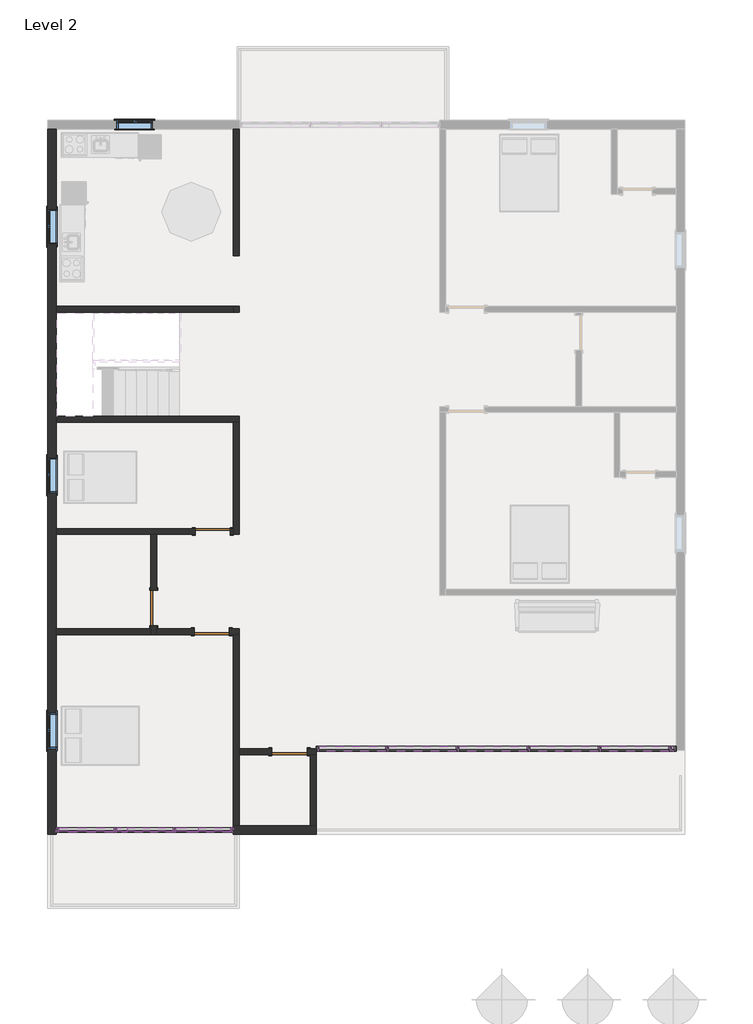
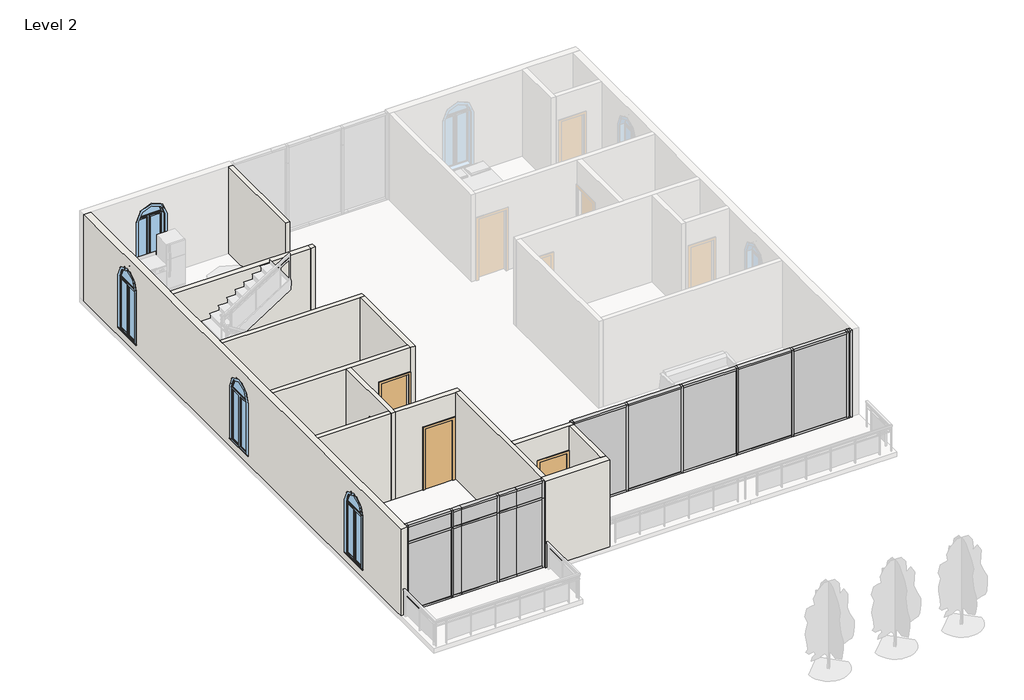
# One storey, part 1 of 3: 42 members, 16 plates, 14 walls, 4 doors, 4 windows.
"""IFC4 building model written with IfcOpenShell, lengths in millimetres."""

from ifc_helpers import new_model, si_unit, frame, origin, place, context, project, spatial, polyline, circle_curve, outline, extrude, faceted_brep, transform, mapped, element, save
from ifc_brep_helpers import plane_surface, revolved_surface, advanced_brep
from components import door_686f89d2, door_16372e1c, member_35f02b64, member_64ee9188, member_6d5c3e5e, member_eaba9652, member_3f395ae9, member_26d67f61, member_f0fea5a5, member_6df10a9f, member_6e77e263, member_ee409385, member_47bfaf8a, member_d2e7e466, member_43f7a5f1, member_c327c56d, member_830eb86c, member_5d67b9fc, member_b5e65c95, member_b3f2e294, member_7db1855a, system_panel_glazed_10fc8cc6, system_panel_glazed_e7b2b8ad, system_panel_glazed_6b5a73aa, system_panel_glazed_adb83807, system_panel_glazed_cd562e5d, system_panel_glazed_a1694ec4, system_panel_glazed_bb2333a0, system_panel_glazed_5dcb8e4e, system_panel_glazed_3760a879, system_panel_glazed_153bb9bb, system_panel_glazed_f2c52b8f, system_panel_glazed_2937bf4c, system_panel_glazed_34036fae, window_e7489165

model = new_model("IFC4")

# Units and contexts
model_context = context("Model", 3, world=origin())
ifc_project = project(units=[si_unit("LENGTHUNIT", "METRE", prefix="MILLI")], contexts=[model_context])

# Site, building, storey
site = spatial("IfcSite", under=ifc_project)
building = spatial("IfcBuilding", under=site)
storey = spatial("IfcBuildingStorey", under=building, Name="Level 2", Elevation=3200.4)

# Doors
placement = place(None, origin())
door_shape = door_686f89d2(model_context)
element("IfcDoor", 1, ObjectType="Single-Flush : 36\" x 84\"", at=placement, inside=storey, context=model_context, shape_type="MappedRepresentation", body=[
    mapped(door_shape, transform((-5050.0707895, -548.4855812, 3200.4), x_axis=(1.0, 0.0, 0.0), y_axis=(0.0, 1.0, 0.0), z_axis=(0.0, 0.0, 1.0))),
])
element("IfcDoor", 2, ObjectType="Single-Flush : 36\" x 84\"", at=placement, inside=storey, context=model_context, shape_type="MappedRepresentation", body=[
    mapped(door_shape, transform((-6548.6707895, 61.1144188, 3200.4), x_axis=(0.0, -1.0, 0.0), y_axis=(1.0, 0.0, 0.0), z_axis=(0.0, 0.0, 1.0))),
])
element("IfcDoor", 3, ObjectType="Single-Flush : 36\" x 84\"", at=placement, inside=storey, context=model_context, shape_type="MappedRepresentation", body=[
    mapped(door_shape, transform((-3043.4707895, -3647.2855812, 3200.4), x_axis=(1.0, 0.0, 0.0), y_axis=(0.0, 1.0, 0.0), z_axis=(0.0, 0.0, 1.0))),
])
door_2_shape = door_16372e1c(model_context)
element("IfcDoor", 4, ObjectType="Single-Flush : 36\" x 84\"", at=placement, inside=storey, context=model_context, shape_type="MappedRepresentation", body=[
    mapped(door_2_shape, transform((-5024.6707895, 2042.3144188, 3200.4), x_axis=(1.0, 0.0, 0.0), y_axis=(0.0, 1.0, 0.0), z_axis=(0.0, 0.0, 1.0))),
])

# Members
member_shape = member_35f02b64(model_context)
element("IfcMember", 5, ObjectType="Rectangular Mullion : 2.5\" x 5\" rectangular", at=placement, inside=storey, context=model_context, shape_type="MappedRepresentation", body=[
    mapped(member_shape, transform((6875.2292105, -3571.0855812, 6248.4), x_axis=(0.0, 0.0, 1.0), y_axis=(0.0, -1.0, 0.0), z_axis=(1.0, 0.0, 0.0))),
])
member_2_shape = member_64ee9188(model_context)
element("IfcMember", 6, ObjectType="Rectangular Mullion : 2.5\" x 5\" rectangular", at=placement, inside=storey, context=model_context, shape_type="MappedRepresentation", body=[
    mapped(member_2_shape, transform((-560.6207895, -3571.0855812, 6248.4), x_axis=(0.0, 0.0, 1.0), y_axis=(0.0, -1.0, 0.0), z_axis=(1.0, 0.0, 0.0))),
])
member_3_shape = member_6d5c3e5e(model_context)
element("IfcMember", 7, ObjectType="Rectangular Mullion : 2.5\" x 5\" rectangular", at=placement, inside=storey, context=model_context, shape_type="MappedRepresentation", body=[
    mapped(member_3_shape, transform((1268.1792105, -3571.0855812, 6248.4), x_axis=(0.0, 0.0, 1.0), y_axis=(0.0, -1.0, 0.0), z_axis=(1.0, 0.0, 0.0))),
])
element("IfcMember", 8, ObjectType="Rectangular Mullion : 2.5\" x 5\" rectangular", at=placement, inside=storey, context=model_context, shape_type="MappedRepresentation", body=[
    mapped(member_3_shape, transform((3096.9792105, -3571.0855812, 6248.4), x_axis=(0.0, 0.0, 1.0), y_axis=(0.0, -1.0, 0.0), z_axis=(1.0, 0.0, 0.0))),
])
element("IfcMember", 9, ObjectType="Rectangular Mullion : 2.5\" x 5\" rectangular", at=placement, inside=storey, context=model_context, shape_type="MappedRepresentation", body=[
    mapped(member_3_shape, transform((4925.7792105, -3571.0855812, 6248.4), x_axis=(0.0, 0.0, 1.0), y_axis=(0.0, -1.0, 0.0), z_axis=(1.0, 0.0, 0.0))),
])
element("IfcMember", 10, ObjectType="Rectangular Mullion : 2.5\" x 5\" rectangular", at=placement, inside=storey, context=model_context, shape_type="MappedRepresentation", body=[
    mapped(member_3_shape, transform((6754.5792105, -3571.0855812, 6248.4), x_axis=(0.0, 0.0, 1.0), y_axis=(0.0, -1.0, 0.0), z_axis=(1.0, 0.0, 0.0))),
])
element("IfcMember", 11, ObjectType="Rectangular Mullion : 2.5\" x 5\" rectangular", at=placement, inside=storey, context=model_context, shape_type="MappedRepresentation", body=[
    mapped(member_2_shape, transform((-2294.1707895, -3571.0855812, 3200.4), x_axis=(0.0, 0.0, -1.0), y_axis=(0.0, -1.0, 0.0), z_axis=(-1.0, 0.0, 0.0))),
])
element("IfcMember", 12, ObjectType="Rectangular Mullion : 2.5\" x 5\" rectangular", at=placement, inside=storey, context=model_context, shape_type="MappedRepresentation", body=[
    mapped(member_3_shape, transform((-497.1207895, -3571.0855812, 3200.4), x_axis=(0.0, 0.0, -1.0), y_axis=(0.0, -1.0, 0.0), z_axis=(-1.0, 0.0, 0.0))),
])
element("IfcMember", 13, ObjectType="Rectangular Mullion : 2.5\" x 5\" rectangular", at=placement, inside=storey, context=model_context, shape_type="MappedRepresentation", body=[
    mapped(member_3_shape, transform((1331.6792105, -3571.0855812, 3200.4), x_axis=(0.0, 0.0, -1.0), y_axis=(0.0, -1.0, 0.0), z_axis=(-1.0, 0.0, 0.0))),
])
element("IfcMember", 14, ObjectType="Rectangular Mullion : 2.5\" x 5\" rectangular", at=placement, inside=storey, context=model_context, shape_type="MappedRepresentation", body=[
    mapped(member_3_shape, transform((3160.4792105, -3571.0855812, 3200.4), x_axis=(0.0, 0.0, -1.0), y_axis=(0.0, -1.0, 0.0), z_axis=(-1.0, 0.0, 0.0))),
])
element("IfcMember", 15, ObjectType="Rectangular Mullion : 2.5\" x 5\" rectangular", at=placement, inside=storey, context=model_context, shape_type="MappedRepresentation", body=[
    mapped(member_3_shape, transform((4989.2792105, -3571.0855812, 3200.4), x_axis=(0.0, 0.0, -1.0), y_axis=(0.0, -1.0, 0.0), z_axis=(-1.0, 0.0, 0.0))),
])
element("IfcMember", 16, ObjectType="Rectangular Mullion : 2.5\" x 5\" rectangular", at=placement, inside=storey, context=model_context, shape_type="MappedRepresentation", body=[
    mapped(member_shape, transform((6818.0792105, -3571.0855812, 3200.4), x_axis=(0.0, 0.0, -1.0), y_axis=(0.0, -1.0, 0.0), z_axis=(-1.0, 0.0, 0.0))),
])
member_4_shape = member_eaba9652(model_context)
element("IfcMember", 17, ObjectType="Rectangular Mullion : 2.5\" x 5\" rectangular", at=placement, inside=storey, context=model_context, shape_type="MappedRepresentation", body=[
    mapped(member_4_shape, transform((-528.8707895, -3571.0855812, 3200.4), x_axis=(1.0, 0.0, 0.0), y_axis=(0.0, -1.0, 0.0), z_axis=(0.0, 0.0, -1.0))),
])
element("IfcMember", 18, ObjectType="Rectangular Mullion : 2.5\" x 5\" rectangular", at=placement, inside=storey, context=model_context, shape_type="MappedRepresentation", body=[
    mapped(member_4_shape, transform((1299.9292105, -3571.0855812, 3200.4), x_axis=(1.0, 0.0, 0.0), y_axis=(0.0, -1.0, 0.0), z_axis=(0.0, 0.0, -1.0))),
])
element("IfcMember", 19, ObjectType="Rectangular Mullion : 2.5\" x 5\" rectangular", at=placement, inside=storey, context=model_context, shape_type="MappedRepresentation", body=[
    mapped(member_4_shape, transform((3128.7292105, -3571.0855812, 3200.4), x_axis=(1.0, 0.0, 0.0), y_axis=(0.0, -1.0, 0.0), z_axis=(0.0, 0.0, -1.0))),
])
element("IfcMember", 20, ObjectType="Rectangular Mullion : 2.5\" x 5\" rectangular", at=placement, inside=storey, context=model_context, shape_type="MappedRepresentation", body=[
    mapped(member_4_shape, transform((4957.5292105, -3571.0855812, 3200.4), x_axis=(1.0, 0.0, 0.0), y_axis=(0.0, -1.0, 0.0), z_axis=(0.0, 0.0, -1.0))),
])
element("IfcMember", 21, ObjectType="Rectangular Mullion : 2.5\" x 5\" rectangular", at=placement, inside=storey, context=model_context, shape_type="MappedRepresentation", body=[
    mapped(member_4_shape, transform((6786.3292105, -3571.0855812, 3200.4), x_axis=(1.0, 0.0, 0.0), y_axis=(0.0, -1.0, 0.0), z_axis=(0.0, 0.0, -1.0))),
])
member_5_shape = member_3f395ae9(model_context)
element("IfcMember", 22, ObjectType="Rectangular Mullion : 2.5\" x 5\" rectangular", at=placement, inside=storey, context=model_context, shape_type="MappedRepresentation", body=[
    mapped(member_5_shape, transform((6938.7292105, -3571.0855812, 3200.4), x_axis=(1.0, 0.0, 0.0), y_axis=(0.0, -1.0, 0.0), z_axis=(0.0, 0.0, -1.0))),
])
element("IfcMember", 23, ObjectType="Rectangular Mullion : 2.5\" x 5\" rectangular", at=placement, inside=storey, context=model_context, shape_type="MappedRepresentation", body=[
    mapped(member_5_shape, transform((-2357.6707895, -3571.0855812, 6248.4), x_axis=(-1.0, 0.0, 0.0), y_axis=(0.0, -1.0, 0.0), z_axis=(0.0, 0.0, 1.0))),
])
member_6_shape = member_26d67f61(model_context)
element("IfcMember", 24, ObjectType="Rectangular Mullion : 2.5\" x 5\" rectangular", at=placement, inside=storey, context=model_context, shape_type="MappedRepresentation", body=[
    mapped(member_6_shape, transform((-8999.7707895, -5666.5046952, 3200.4), x_axis=(0.0, 0.0, -1.0), y_axis=(0.0, -1.0, 0.0), z_axis=(-1.0, 0.0, 0.0))),
])
element("IfcMember", 25, ObjectType="Rectangular Mullion : 2.5\" x 5\" rectangular", at=placement, inside=storey, context=model_context, shape_type="MappedRepresentation", body=[
    mapped(member_6_shape, transform((-7571.0207895, -5666.5046952, 6248.4), x_axis=(0.0, 0.0, 1.0), y_axis=(0.0, -1.0, 0.0), z_axis=(1.0, 0.0, 0.0))),
])
member_7_shape = member_f0fea5a5(model_context)
element("IfcMember", 26, ObjectType="Rectangular Mullion : 2.5\" x 5\" rectangular", at=placement, inside=storey, context=model_context, shape_type="MappedRepresentation", body=[
    mapped(member_7_shape, transform((-7539.2707895, -5666.5046952, 3200.4), x_axis=(1.0, 0.0, 0.0), y_axis=(0.0, -1.0, 0.0), z_axis=(0.0, 0.0, -1.0))),
])
element("IfcMember", 27, ObjectType="Rectangular Mullion : 2.5\" x 5\" rectangular", at=placement, inside=storey, context=model_context, shape_type="MappedRepresentation", body=[
    mapped(member_7_shape, transform((-6015.2707895, -5666.5046952, 3200.4), x_axis=(1.0, 0.0, 0.0), y_axis=(0.0, -1.0, 0.0), z_axis=(0.0, 0.0, -1.0))),
])
member_8_shape = member_6df10a9f(model_context)
element("IfcMember", 28, ObjectType="Rectangular Mullion : 2.5\" x 5\" rectangular", at=placement, inside=storey, context=model_context, shape_type="MappedRepresentation", body=[
    mapped(member_8_shape, transform((-7571.0207895, -5666.5046952, 5638.8), x_axis=(0.0, 0.0, 1.0), y_axis=(0.0, -1.0, 0.0), z_axis=(1.0, 0.0, 0.0))),
])
member_9_shape = member_6e77e263(model_context)
element("IfcMember", 29, ObjectType="Rectangular Mullion : 2.5\" x 5\" rectangular", at=placement, inside=storey, context=model_context, shape_type="MappedRepresentation", body=[
    mapped(member_9_shape, transform((-7539.2707895, -5666.5046952, 5638.8), x_axis=(1.0, 0.0, 0.0), y_axis=(0.0, -1.0, 0.0), z_axis=(0.0, 0.0, -1.0))),
])
element("IfcMember", 30, ObjectType="Rectangular Mullion : 2.5\" x 5\" rectangular", at=placement, inside=storey, context=model_context, shape_type="MappedRepresentation", body=[
    mapped(member_9_shape, transform((-6015.2707895, -5666.5046952, 5638.8), x_axis=(1.0, 0.0, 0.0), y_axis=(0.0, -1.0, 0.0), z_axis=(0.0, 0.0, -1.0))),
])
member_10_shape = member_ee409385(model_context)
element("IfcMember", 31, ObjectType="Rectangular Mullion : 2.5\" x 5\" rectangular", at=placement, inside=storey, context=model_context, shape_type="MappedRepresentation", body=[
    mapped(member_10_shape, transform((-4491.2707895, -5666.5046952, 3200.4), x_axis=(1.0, 0.0, 0.0), y_axis=(0.0, -1.0, 0.0), z_axis=(0.0, 0.0, -1.0))),
])
member_11_shape = member_47bfaf8a(model_context)
element("IfcMember", 32, ObjectType="Rectangular Mullion : 2.5\" x 5\" rectangular", at=placement, inside=storey, context=model_context, shape_type="MappedRepresentation", body=[
    mapped(member_11_shape, transform((-9063.2707895, -5666.5046952, 6248.4), x_axis=(-1.0, 0.0, 0.0), y_axis=(0.0, -1.0, 0.0), z_axis=(0.0, 0.0, 1.0))),
])
element("IfcMember", 33, ObjectType="Rectangular Mullion : 2.5\" x 5\" rectangular", at=placement, inside=storey, context=model_context, shape_type="MappedRepresentation", body=[
    mapped(member_11_shape, transform((-4491.2707895, -5666.5046952, 5638.8), x_axis=(1.0, 0.0, 0.0), y_axis=(0.0, -1.0, 0.0), z_axis=(0.0, 0.0, -1.0))),
])
element("IfcMember", 34, ObjectType="Rectangular Mullion : 2.5\" x 5\" rectangular", at=placement, inside=storey, context=model_context, shape_type="MappedRepresentation", body=[
    mapped(member_10_shape, transform((-9063.2707895, -5666.5046952, 5638.8), x_axis=(-1.0, 0.0, 0.0), y_axis=(0.0, -1.0, 0.0), z_axis=(0.0, 0.0, 1.0))),
])
member_12_shape = member_d2e7e466(model_context)
element("IfcMember", 35, ObjectType="Rectangular Mullion : 2.5\" x 5\" rectangular", at=placement, inside=storey, context=model_context, shape_type="MappedRepresentation", body=[
    mapped(member_12_shape, transform((-4554.7707895, -5666.5046952, 6248.4), x_axis=(0.0, 0.0, 1.0), y_axis=(0.0, -1.0, 0.0), z_axis=(1.0, 0.0, 0.0))),
])
member_13_shape = member_43f7a5f1(model_context)
element("IfcMember", 36, ObjectType="Rectangular Mullion : 2.5\" x 5\" rectangular", at=placement, inside=storey, context=model_context, shape_type="MappedRepresentation", body=[
    mapped(member_13_shape, transform((-6047.0207895, -5666.5046952, 6248.4), x_axis=(0.0, 0.0, 1.0), y_axis=(0.0, -1.0, 0.0), z_axis=(1.0, 0.0, 0.0))),
])
member_14_shape = member_c327c56d(model_context)
element("IfcMember", 37, ObjectType="Rectangular Mullion : 2.5\" x 5\" rectangular", at=placement, inside=storey, context=model_context, shape_type="MappedRepresentation", body=[
    mapped(member_14_shape, transform((-7507.5207895, -5666.5046952, 3200.4), x_axis=(0.0, 0.0, -1.0), y_axis=(0.0, -1.0, 0.0), z_axis=(-1.0, 0.0, 0.0))),
])
member_15_shape = member_830eb86c(model_context)
element("IfcMember", 38, ObjectType="Rectangular Mullion : 2.5\" x 5\" rectangular", at=placement, inside=storey, context=model_context, shape_type="MappedRepresentation", body=[
    mapped(member_15_shape, transform((-5983.5207895, -5666.5046952, 3200.4), x_axis=(0.0, 0.0, -1.0), y_axis=(0.0, -1.0, 0.0), z_axis=(-1.0, 0.0, 0.0))),
])
member_16_shape = member_5d67b9fc(model_context)
element("IfcMember", 39, ObjectType="Rectangular Mullion : 2.5\" x 5\" rectangular", at=placement, inside=storey, context=model_context, shape_type="MappedRepresentation", body=[
    mapped(member_16_shape, transform((-7234.4707895, -5666.5046952, 5638.8), x_axis=(0.0, 0.0, 1.0), y_axis=(0.0, -1.0, 0.0), z_axis=(1.0, 0.0, 0.0))),
])
member_17_shape = member_b5e65c95(model_context)
element("IfcMember", 40, ObjectType="Rectangular Mullion : 2.5\" x 5\" rectangular", at=placement, inside=storey, context=model_context, shape_type="MappedRepresentation", body=[
    mapped(member_17_shape, transform((-5405.6707895, -5666.5046952, 5638.8), x_axis=(0.0, 0.0, 1.0), y_axis=(0.0, -1.0, 0.0), z_axis=(1.0, 0.0, 0.0))),
])
element("IfcMember", 41, ObjectType="Rectangular Mullion : 2.5\" x 5\" rectangular", at=placement, inside=storey, context=model_context, shape_type="MappedRepresentation", body=[
    mapped(member_15_shape, transform((-5405.6707895, -5666.5046952, 6248.4), x_axis=(0.0, 0.0, 1.0), y_axis=(0.0, -1.0, 0.0), z_axis=(1.0, 0.0, 0.0))),
])
element("IfcMember", 42, ObjectType="Rectangular Mullion : 2.5\" x 5\" rectangular", at=placement, inside=storey, context=model_context, shape_type="MappedRepresentation", body=[
    mapped(member_14_shape, transform((-7234.4707895, -5666.5046952, 6248.4), x_axis=(0.0, 0.0, 1.0), y_axis=(0.0, -1.0, 0.0), z_axis=(1.0, 0.0, 0.0))),
])
element("IfcMember", 43, ObjectType="Rectangular Mullion : 2.5\" x 5\" rectangular", at=placement, inside=storey, context=model_context, shape_type="MappedRepresentation", body=[
    mapped(member_13_shape, transform((-7234.4707895, -5666.5046952, 3200.4), x_axis=(0.0, 0.0, -1.0), y_axis=(0.0, -1.0, 0.0), z_axis=(-1.0, 0.0, 0.0))),
])
element("IfcMember", 44, ObjectType="Rectangular Mullion : 2.5\" x 5\" rectangular", at=placement, inside=storey, context=model_context, shape_type="MappedRepresentation", body=[
    mapped(member_12_shape, transform((-5405.6707895, -5666.5046952, 3200.4), x_axis=(0.0, 0.0, -1.0), y_axis=(0.0, -1.0, 0.0), z_axis=(-1.0, 0.0, 0.0))),
])
member_18_shape = member_b3f2e294(model_context)
element("IfcMember", 45, ObjectType="Rectangular Mullion : 2.5\" x 5\" rectangular", at=placement, inside=storey, context=model_context, shape_type="MappedRepresentation", body=[
    mapped(member_18_shape, transform((-6047.0207895, -5666.5046952, 5638.8), x_axis=(0.0, 0.0, 1.0), y_axis=(0.0, -1.0, 0.0), z_axis=(1.0, 0.0, 0.0))),
])
member_19_shape = member_7db1855a(model_context)
element("IfcMember", 46, ObjectType="Rectangular Mullion : 2.5\" x 5\" rectangular", at=placement, inside=storey, context=model_context, shape_type="MappedRepresentation", body=[
    mapped(member_19_shape, transform((-4554.7707895, -5666.5046952, 5638.8), x_axis=(0.0, 0.0, 1.0), y_axis=(0.0, -1.0, 0.0), z_axis=(1.0, 0.0, 0.0))),
])

# Plates
system_panel_glazed_shape = system_panel_glazed_10fc8cc6(model_context)
element("IfcPlate", 47, ObjectType="System Panel : Glazed", at=placement, inside=storey, context=model_context, shape_type="MappedRepresentation", body=[
    mapped(system_panel_glazed_shape, transform((385.5292105, -3571.0855812, 3263.9), x_axis=(1.0, 0.0, 0.0), y_axis=(0.0, 1.0, 0.0), z_axis=(0.0, 0.0, 1.0))),
])
element("IfcPlate", 48, ObjectType="System Panel : Glazed", at=placement, inside=storey, context=model_context, shape_type="MappedRepresentation", body=[
    mapped(system_panel_glazed_shape, transform((2214.3292105, -3571.0855812, 3263.9), x_axis=(1.0, 0.0, 0.0), y_axis=(0.0, 1.0, 0.0), z_axis=(0.0, 0.0, 1.0))),
])
element("IfcPlate", 49, ObjectType="System Panel : Glazed", at=placement, inside=storey, context=model_context, shape_type="MappedRepresentation", body=[
    mapped(system_panel_glazed_shape, transform((4043.1292105, -3571.0855812, 3263.9), x_axis=(1.0, 0.0, 0.0), y_axis=(0.0, 1.0, 0.0), z_axis=(0.0, 0.0, 1.0))),
])
element("IfcPlate", 50, ObjectType="System Panel : Glazed", at=placement, inside=storey, context=model_context, shape_type="MappedRepresentation", body=[
    mapped(system_panel_glazed_shape, transform((5871.9292105, -3571.0855812, 3263.9), x_axis=(1.0, 0.0, 0.0), y_axis=(0.0, 1.0, 0.0), z_axis=(0.0, 0.0, 1.0))),
])
system_panel_glazed_2_shape = system_panel_glazed_e7b2b8ad(model_context)
element("IfcPlate", 51, ObjectType="System Panel : Glazed", at=placement, inside=storey, context=model_context, shape_type="MappedRepresentation", body=[
    mapped(system_panel_glazed_2_shape, transform((6846.6542105, -3571.0855812, 3263.9), x_axis=(1.0, 0.0, 0.0), y_axis=(0.0, 1.0, 0.0), z_axis=(0.0, 0.0, 1.0))),
])
system_panel_glazed_3_shape = system_panel_glazed_6b5a73aa(model_context)
element("IfcPlate", 52, ObjectType="System Panel : Glazed", at=placement, inside=storey, context=model_context, shape_type="MappedRepresentation", body=[
    mapped(system_panel_glazed_3_shape, transform((-1427.3957895, -3571.0855812, 3263.9), x_axis=(1.0, 0.0, 0.0), y_axis=(0.0, 1.0, 0.0), z_axis=(0.0, 0.0, 1.0))),
])
system_panel_glazed_4_shape = system_panel_glazed_adb83807(model_context)
element("IfcPlate", 53, ObjectType="System Panel : Glazed", at=placement, inside=storey, context=model_context, shape_type="MappedRepresentation", body=[
    mapped(system_panel_glazed_4_shape, transform((-8285.3957895, -5666.5046952, 3263.9), x_axis=(1.0, 0.0, 0.0), y_axis=(0.0, 1.0, 0.0), z_axis=(0.0, 0.0, 1.0))),
])
system_panel_glazed_5_shape = system_panel_glazed_cd562e5d(model_context)
element("IfcPlate", 54, ObjectType="System Panel : Glazed", at=placement, inside=storey, context=model_context, shape_type="MappedRepresentation", body=[
    mapped(system_panel_glazed_5_shape, transform((-8285.3957895, -5666.5046952, 5670.55), x_axis=(1.0, 0.0, 0.0), y_axis=(0.0, 1.0, 0.0), z_axis=(0.0, 0.0, 1.0))),
])
system_panel_glazed_6_shape = system_panel_glazed_a1694ec4(model_context)
element("IfcPlate", 55, ObjectType="System Panel : Glazed", at=placement, inside=storey, context=model_context, shape_type="MappedRepresentation", body=[
    mapped(system_panel_glazed_6_shape, transform((-7370.9957895, -5666.5046952, 3263.9), x_axis=(1.0, 0.0, 0.0), y_axis=(0.0, 1.0, 0.0), z_axis=(0.0, 0.0, 1.0))),
])
system_panel_glazed_7_shape = system_panel_glazed_bb2333a0(model_context)
element("IfcPlate", 56, ObjectType="System Panel : Glazed", at=placement, inside=storey, context=model_context, shape_type="MappedRepresentation", body=[
    mapped(system_panel_glazed_7_shape, transform((-5694.5957895, -5666.5046952, 3263.9), x_axis=(1.0, 0.0, 0.0), y_axis=(0.0, 1.0, 0.0), z_axis=(0.0, 0.0, 1.0))),
])
system_panel_glazed_8_shape = system_panel_glazed_5dcb8e4e(model_context)
element("IfcPlate", 57, ObjectType="System Panel : Glazed", at=placement, inside=storey, context=model_context, shape_type="MappedRepresentation", body=[
    mapped(system_panel_glazed_8_shape, transform((-7370.9957895, -5666.5046952, 5670.55), x_axis=(1.0, 0.0, 0.0), y_axis=(0.0, 1.0, 0.0), z_axis=(0.0, 0.0, 1.0))),
])
system_panel_glazed_9_shape = system_panel_glazed_3760a879(model_context)
element("IfcPlate", 58, ObjectType="System Panel : Glazed", at=placement, inside=storey, context=model_context, shape_type="MappedRepresentation", body=[
    mapped(system_panel_glazed_9_shape, transform((-5694.5957895, -5666.5046952, 5670.55), x_axis=(1.0, 0.0, 0.0), y_axis=(0.0, 1.0, 0.0), z_axis=(0.0, 0.0, 1.0))),
])
system_panel_glazed_10_shape = system_panel_glazed_153bb9bb(model_context)
element("IfcPlate", 59, ObjectType="System Panel : Glazed", at=placement, inside=storey, context=model_context, shape_type="MappedRepresentation", body=[
    mapped(system_panel_glazed_10_shape, transform((-6640.7457895, -5666.5046952, 3263.9), x_axis=(1.0, 0.0, 0.0), y_axis=(0.0, 1.0, 0.0), z_axis=(0.0, 0.0, 1.0))),
])
system_panel_glazed_11_shape = system_panel_glazed_f2c52b8f(model_context)
element("IfcPlate", 60, ObjectType="System Panel : Glazed", at=placement, inside=storey, context=model_context, shape_type="MappedRepresentation", body=[
    mapped(system_panel_glazed_11_shape, transform((-6640.7457895, -5666.5046952, 5670.55), x_axis=(1.0, 0.0, 0.0), y_axis=(0.0, 1.0, 0.0), z_axis=(0.0, 0.0, 1.0))),
])
system_panel_glazed_12_shape = system_panel_glazed_2937bf4c(model_context)
element("IfcPlate", 61, ObjectType="System Panel : Glazed", at=placement, inside=storey, context=model_context, shape_type="MappedRepresentation", body=[
    mapped(system_panel_glazed_12_shape, transform((-4980.2207895, -5666.5046952, 3263.9), x_axis=(1.0, 0.0, 0.0), y_axis=(0.0, 1.0, 0.0), z_axis=(0.0, 0.0, 1.0))),
])
system_panel_glazed_13_shape = system_panel_glazed_34036fae(model_context)
element("IfcPlate", 62, ObjectType="System Panel : Glazed", at=placement, inside=storey, context=model_context, shape_type="MappedRepresentation", body=[
    mapped(system_panel_glazed_13_shape, transform((-4980.2207895, -5666.5046952, 5670.55), x_axis=(1.0, 0.0, 0.0), y_axis=(0.0, 1.0, 0.0), z_axis=(0.0, 0.0, 1.0))),
])

# Walls
element("IfcWall", 63, ObjectType="6\"", at=placement, inside=storey, context=model_context, shape_type="SweptSolid", body=[
    extrude(outline(polyline([(-4491.2707895, 9167.0144188), (-4491.2707895, 12430.9144188), (-4338.8707895, 12430.9144188), (-4338.8707895, 9167.0144188), (-4491.2707895, 9167.0144188)])), frame((0.0, 0.0, 3200.4), z_axis=(0.0, 0.0, 1.0), x_axis=(1.0, 0.0, 0.0)), (0.0, 0.0, 1.0), 3048.0),
])
element("IfcWall", 64, ObjectType="6\"", at=placement, inside=storey, context=model_context, shape_type="SweptSolid", body=[
    extrude(outline(polyline([(-9063.2707895, 7858.9144188), (-4491.2707895, 7858.9144188), (-4491.2707895, 7706.5144188), (-9063.2707895, 7706.5144188), (-9063.2707895, 7858.9144188)])), frame((0.0, 0.0, 3200.4), z_axis=(0.0, 0.0, 1.0), x_axis=(1.0, 0.0, 0.0)), (0.0, 0.0, 1.0), 3048.0),
])
element("IfcWall", 65, ObjectType="6\"", at=placement, inside=storey, context=model_context, shape_type="Brep", body=[
    faceted_brep([(-9063.2707895, 4861.7144188, 3200.4), (-4491.2707895, 4861.7144188, 3200.4), (-4338.8707895, 4861.7144188, 3200.4), (-4338.8707895, 4861.7144188, 6248.4), (-4491.2707895, 4861.7144188, 6248.4), (-9063.2707895, 4861.7144188, 6248.4), (-9063.2707895, 5014.1144188, 3200.4), (-9063.2707895, 5014.1144188, 6248.4), (-4338.8707895, 5014.1144188, 6248.4), (-4338.8707895, 5014.1144188, 3200.4)], [[[0, 1, 2, 3, 4, 5]], [[6, 7, 8, 9]], [[2, 1, 0, 6, 9]], [[5, 4, 3, 8, 7]], [[3, 2, 9, 8]], [[0, 5, 7, 6]]]),
])
element("IfcWall", 66, ObjectType="6\"", at=placement, inside=storey, context=model_context, shape_type="Brep", body=[
    faceted_brep([(-4491.2707895, 4861.7144188, 3200.4), (-4491.2707895, 2118.5144188, 3200.4), (-4491.2707895, 1966.1144188, 3200.4), (-4491.2707895, 1966.1144188, 6248.4), (-4491.2707895, 2118.5144188, 6248.4), (-4491.2707895, 4861.7144188, 6248.4), (-4338.8707895, 4861.7144188, 3200.4), (-4338.8707895, 4861.7144188, 6248.4), (-4338.8707895, 1966.1144188, 6248.4), (-4338.8707895, 1966.1144188, 3200.4)], [[[0, 1, 2, 3, 4, 5]], [[6, 7, 8, 9]], [[2, 1, 0, 6, 9]], [[5, 4, 3, 8, 7]], [[0, 5, 7, 6]], [[3, 2, 9, 8]]]),
])
element("IfcWall", 67, ObjectType="6\"", at=placement, inside=storey, context=model_context, shape_type="Brep", body=[
    faceted_brep([(-4491.2707895, 2118.5144188, 3200.4), (-4567.4707895, 2118.5144188, 3200.4), (-4567.4707895, 2118.5144188, 5334.0), (-5481.8707895, 2118.5144188, 5334.0), (-5481.8707895, 2118.5144188, 3200.4), (-9063.2707895, 2118.5144188, 3200.4), (-9063.2707895, 2118.5144188, 6248.4), (-4491.2707895, 2118.5144188, 6248.4), (-4567.4707895, 1966.1144188, 5334.0), (-4567.4707895, 1966.1144188, 3200.4), (-4491.2707895, 1966.1144188, 3200.4), (-4491.2707895, 1966.1144188, 6248.4), (-6472.4707895, 1966.1144188, 6248.4), (-6624.8707895, 1966.1144188, 6248.4), (-9063.2707895, 1966.1144188, 6248.4), (-9063.2707895, 1966.1144188, 3200.4), (-6624.8707895, 1966.1144188, 3200.4), (-6472.4707895, 1966.1144188, 3200.4), (-5481.8707895, 1966.1144188, 3200.4), (-5481.8707895, 1966.1144188, 5334.0)], [[[0, 1, 2, 3, 4, 5, 6, 7]], [[8, 9, 10, 11, 12, 13, 14, 15, 16, 17, 18, 19]], [[10, 9, 1, 0]], [[18, 17, 16, 15, 5, 4]], [[7, 6, 14, 13, 12, 11]], [[0, 7, 11, 10]], [[6, 5, 15, 14]], [[2, 1, 9, 8]], [[3, 2, 8, 19]], [[4, 3, 19, 18]]]),
])
element("IfcWall", 68, ObjectType="6\"", at=placement, inside=storey, context=model_context, shape_type="Brep", body=[
    faceted_brep([(-6624.8707895, -396.0855812, 5334.0), (-6624.8707895, -396.0855812, 3200.4), (-6624.8707895, -472.2855812, 3200.4), (-6624.8707895, -624.6855812, 3200.4), (-6624.8707895, -624.6855812, 6248.4), (-6624.8707895, -472.2855812, 6248.4), (-6624.8707895, 1966.1144188, 6248.4), (-6624.8707895, 1966.1144188, 3200.4), (-6624.8707895, 518.3144188, 3200.4), (-6624.8707895, 518.3144188, 5334.0), (-6472.4707895, -624.6855812, 3200.4), (-6472.4707895, -472.2855812, 3200.4), (-6472.4707895, -396.0855812, 3200.4), (-6472.4707895, -396.0855812, 5334.0), (-6472.4707895, 518.3144188, 5334.0), (-6472.4707895, 518.3144188, 3200.4), (-6472.4707895, 1966.1144188, 3200.4), (-6472.4707895, 1966.1144188, 6248.4), (-6472.4707895, -472.2855812, 6248.4), (-6472.4707895, -624.6855812, 6248.4)], [[[0, 1, 2, 3, 4, 5, 6, 7, 8, 9]], [[10, 11, 12, 13, 14, 15, 16, 17, 18, 19]], [[8, 7, 16, 15]], [[3, 2, 1, 12, 11, 10]], [[6, 5, 4, 19, 18, 17]], [[7, 6, 17, 16]], [[4, 3, 10, 19]], [[13, 12, 1, 0]], [[14, 13, 0, 9]], [[15, 14, 9, 8]]]),
])
element("IfcWall", 69, ObjectType="6\"", at=placement, inside=storey, context=model_context, shape_type="SweptSolid", body=[
    extrude(outline(polyline([(-9063.2707895, -472.2855812), (-6624.8707895, -472.2855812), (-6624.8707895, -624.6855812), (-9063.2707895, -624.6855812), (-9063.2707895, -472.2855812)])), frame((0.0, 0.0, 3200.4), z_axis=(0.0, 0.0, 1.0), x_axis=(1.0, 0.0, 0.0)), (0.0, 0.0, 1.0), 3048.0),
])
element("IfcWall", 70, ObjectType="6\"", at=placement, inside=storey, context=model_context, shape_type="Brep", body=[
    faceted_brep([(-4592.8707895, -624.6855812, 5334.0), (-4592.8707895, -624.6855812, 3200.4), (-4491.2707895, -624.6855812, 3200.4), (-4338.8707895, -624.6855812, 3200.4), (-4338.8707895, -624.6855812, 6248.4), (-4491.2707895, -624.6855812, 6248.4), (-6472.4707895, -624.6855812, 6248.4), (-6472.4707895, -624.6855812, 3200.4), (-5507.2707895, -624.6855812, 3200.4), (-5507.2707895, -624.6855812, 5334.0), (-4338.8707895, -472.2855812, 3200.4), (-4592.8707895, -472.2855812, 3200.4), (-4592.8707895, -472.2855812, 5334.0), (-5507.2707895, -472.2855812, 5334.0), (-5507.2707895, -472.2855812, 3200.4), (-6472.4707895, -472.2855812, 3200.4), (-6472.4707895, -472.2855812, 6248.4), (-4338.8707895, -472.2855812, 6248.4)], [[[0, 1, 2, 3, 4, 5, 6, 7, 8, 9]], [[10, 11, 12, 13, 14, 15, 16, 17]], [[8, 7, 15, 14]], [[3, 2, 1, 11, 10]], [[6, 5, 4, 17, 16]], [[7, 6, 16, 15]], [[4, 3, 10, 17]], [[12, 11, 1, 0]], [[13, 12, 0, 9]], [[14, 13, 9, 8]]]),
])
element("IfcWall", 71, ObjectType="6\"", at=placement, inside=storey, context=model_context, shape_type="Brep", body=[
    faceted_brep([(-4491.2707895, -624.6855812, 3200.4), (-4491.2707895, -5552.2855812, 3200.4), (-4491.2707895, -5552.2855812, 6248.4), (-4491.2707895, -624.6855812, 6248.4), (-4338.8707895, -624.6855812, 3200.4), (-4338.8707895, -624.6855812, 6248.4), (-4338.8707895, -3571.0855812, 6248.4), (-4338.8707895, -3723.4855812, 6248.4), (-4338.8707895, -5552.2855812, 6248.4), (-4338.8707895, -5552.2855812, 3200.4), (-4338.8707895, -3723.4855812, 3200.4), (-4338.8707895, -3571.0855812, 3200.4)], [[[0, 1, 2, 3]], [[4, 5, 6, 7, 8, 9, 10, 11]], [[1, 0, 4, 11, 10, 9]], [[3, 2, 8, 7, 6, 5]], [[0, 3, 5, 4]], [[2, 1, 9, 8]]]),
])
element("IfcWall", 72, ObjectType="6\"", at=placement, inside=storey, context=model_context, shape_type="Brep", body=[
    faceted_brep([(-2586.2707895, -3723.4855812, 5334.0), (-2586.2707895, -3723.4855812, 3200.4), (-2510.0707895, -3723.4855812, 3200.4), (-2357.6707895, -3723.4855812, 3200.4), (-2357.6707895, -3723.4855812, 6248.4), (-2510.0707895, -3723.4855812, 6248.4), (-4338.8707895, -3723.4855812, 6248.4), (-4338.8707895, -3723.4855812, 3200.4), (-3500.6707895, -3723.4855812, 3200.4), (-3500.6707895, -3723.4855812, 5334.0), (-2357.6707895, -3571.0855812, 3200.4), (-2586.2707895, -3571.0855812, 3200.4), (-2586.2707895, -3571.0855812, 5334.0), (-3500.6707895, -3571.0855812, 5334.0), (-3500.6707895, -3571.0855812, 3200.4), (-4338.8707895, -3571.0855812, 3200.4), (-4338.8707895, -3571.0855812, 6248.4), (-2357.6707895, -3571.0855812, 6248.4)], [[[0, 1, 2, 3, 4, 5, 6, 7, 8, 9]], [[10, 11, 12, 13, 14, 15, 16, 17]], [[8, 7, 15, 14]], [[3, 2, 1, 11, 10]], [[6, 5, 4, 17, 16]], [[7, 6, 16, 15]], [[4, 3, 10, 17]], [[12, 11, 1, 0]], [[13, 12, 0, 9]], [[14, 13, 9, 8]]]),
])
element("IfcWall", 73, ObjectType="6\"", at=placement, inside=storey, context=model_context, shape_type="SweptSolid", body=[
    extrude(outline(polyline([(-2510.0707895, -5552.2855812), (-2510.0707895, -3723.4855812), (-2357.6707895, -3723.4855812), (-2357.6707895, -5552.2855812), (-2510.0707895, -5552.2855812)])), frame((0.0, 0.0, 3200.4), z_axis=(0.0, 0.0, 1.0), x_axis=(1.0, 0.0, 0.0)), (0.0, 0.0, 1.0), 3048.0),
])
element("IfcWall", 74, ObjectType="6\"", at=placement, inside=storey, context=model_context, shape_type="SweptSolid", body=[
    extrude(outline(polyline([(-4491.2707895, 7706.5144188), (-4491.2707895, 7858.9144188), (-4338.8707895, 7858.9144188), (-4338.8707895, 7706.5144188), (-4491.2707895, 7706.5144188)])), frame((0.0, 0.0, 3200.4), z_axis=(0.0, 0.0, 1.0), x_axis=(1.0, 0.0, 0.0)), (0.0, 0.0, 1.0), 3048.0),
])
element("IfcWall", 75, ObjectType="9\"", at=placement, inside=storey, context=model_context, shape_type="AdvancedBrep", body=[
    advanced_brep(
    [(-9291.8707895, 12430.9144188, 3200.4), (-9291.8707895, -5780.8046952, 3200.4), (-9291.8707895, -5780.8046952, 6248.4), (-9291.8707895, 12430.9144188, 6248.4), (-9291.8707895, -2650.3355812, 5353.05), (-9291.8707895, -3564.7355812, 5353.05), (-9291.8707895, -3564.7355812, 3505.2), (-9291.8707895, -2650.3355812, 3505.2), (-9291.8707895, 3947.3144188, 5353.05), (-9291.8707895, 3032.9144188, 5353.05), (-9291.8707895, 3032.9144188, 3505.2), (-9291.8707895, 3947.3144188, 3505.2), (-9291.8707895, 10367.1644188, 5353.05), (-9291.8707895, 9452.7644188, 5353.05), (-9291.8707895, 9452.7644188, 3505.2), (-9291.8707895, 10367.1644188, 3505.2), (-9063.2707895, 12430.9144188, 3200.4), (-9063.2707895, 12430.9144188, 6248.4), (-9063.2707895, 7858.9144188, 6248.4), (-9063.2707895, 7706.5144188, 6248.4), (-9063.2707895, 5014.1144188, 6248.4), (-9063.2707895, 4861.7144188, 6248.4), (-9063.2707895, 2118.5144188, 6248.4), (-9063.2707895, 1966.1144188, 6248.4), (-9063.2707895, -472.2855812, 6248.4), (-9063.2707895, -624.6855812, 6248.4), (-9063.2707895, -5780.8046952, 6248.4), (-9063.2707895, -5780.8046952, 3200.4), (-9063.2707895, -624.6855812, 3200.4), (-9063.2707895, -472.2855812, 3200.4), (-9063.2707895, 1966.1144188, 3200.4), (-9063.2707895, 2118.5144188, 3200.4), (-9063.2707895, 4861.7144188, 3200.4), (-9063.2707895, 5014.1144188, 3200.4), (-9063.2707895, 7706.5144188, 3200.4), (-9063.2707895, 7858.9144188, 3200.4), (-9063.2707895, -2650.3355812, 5353.05), (-9063.2707895, -2650.3355812, 3505.2), (-9063.2707895, -3564.7355812, 3505.2), (-9063.2707895, -3564.7355812, 5353.05), (-9063.2707895, 3947.3144188, 5353.05), (-9063.2707895, 3947.3144188, 3505.2), (-9063.2707895, 3032.9144188, 3505.2), (-9063.2707895, 3032.9144188, 5353.05), (-9063.2707895, 10367.1644188, 5353.05), (-9063.2707895, 10367.1644188, 3505.2), (-9063.2707895, 9452.7644188, 3505.2), (-9063.2707895, 9452.7644188, 5353.05)],
    [
        (0, 1),
        (1, 2),
        (2, 3),
        (3, 0),
        (4, 5, circle_curve(frame((-9291.8707895, -3107.5355812, 5353.05), z_axis=(1.0, 0.0, 0.0), x_axis=(0.0, 1.0, 0.0)), 457.2)),
        (5, 6),
        (6, 7),
        (7, 4),
        (8, 9, circle_curve(frame((-9291.8707895, 3490.1144188, 5353.05), z_axis=(1.0, 0.0, 0.0), x_axis=(0.0, 1.0, 0.0)), 457.2)),
        (9, 10),
        (10, 11),
        (11, 8),
        (12, 13, circle_curve(frame((-9291.8707895, 9909.9644188, 5353.05), z_axis=(1.0, 0.0, 0.0), x_axis=(0.0, 1.0, 0.0)), 457.2)),
        (13, 14),
        (14, 15),
        (15, 12),
        (16, 17),
        (17, 18),
        (18, 19),
        (19, 20),
        (20, 21),
        (21, 22),
        (22, 23),
        (23, 24),
        (24, 25),
        (25, 26),
        (26, 27),
        (27, 28),
        (28, 29),
        (29, 30),
        (30, 31),
        (31, 32),
        (32, 33),
        (33, 34),
        (34, 35),
        (35, 16),
        (36, 37),
        (37, 38),
        (38, 39),
        (39, 36, circle_curve(frame((-9063.2707895, -3107.5355812, 5353.05), z_axis=(-1.0, 0.0, 0.0), x_axis=(0.0, 1.0, 0.0)), 457.2)),
        (40, 41),
        (41, 42),
        (42, 43),
        (43, 40, circle_curve(frame((-9063.2707895, 3490.1144188, 5353.05), z_axis=(-1.0, 0.0, 0.0), x_axis=(0.0, 1.0, 0.0)), 457.2)),
        (44, 45),
        (45, 46),
        (46, 47),
        (47, 44, circle_curve(frame((-9063.2707895, 9909.9644188, 5353.05), z_axis=(-1.0, 0.0, 0.0), x_axis=(0.0, 1.0, 0.0)), 457.2)),
        (0, 16),
        (27, 1),
        (26, 2),
        (17, 3),
        (36, 4),
        (7, 37),
        (6, 38),
        (5, 39),
        (40, 8),
        (11, 41),
        (10, 42),
        (9, 43),
        (44, 12),
        (15, 45),
        (14, 46),
        (13, 47),
    ],
    [
        plane_surface(frame((-9291.8707895, 12430.9144188, 3200.4), z_axis=(-1.0, 0.0, 0.0), x_axis=(0.0, -1.0, 0.0))),
        plane_surface(frame((-9063.2707895, 12430.9144188, 3200.4), z_axis=(1.0, 0.0, 0.0), x_axis=(0.0, 1.0, 0.0))),
        plane_surface(frame((-9291.8707895, 12545.2144188, 3200.4), z_axis=(0.0, 0.0, -1.0), x_axis=(1.0, 0.0, 0.0))),
        plane_surface(frame((-9291.8707895, -5780.8046952, 3200.4), z_axis=(0.0, -1.0, 0.0), x_axis=(1.0, 0.0, 0.0))),
        plane_surface(frame((-9291.8707895, -5780.8046952, 6248.4), z_axis=(0.0, 0.0, 1.0), x_axis=(1.0, 0.0, 0.0))),
        plane_surface(frame((-9063.2707895, -2650.3355812, 5353.05), z_axis=(0.0, -1.0, 0.0), x_axis=(-1.0, 0.0, 0.0))),
        plane_surface(frame((-9063.2707895, -2650.3355812, 3505.2), z_axis=(0.0, 0.0, 1.0), x_axis=(-1.0, 0.0, 0.0))),
        plane_surface(frame((-9063.2707895, -3564.7355812, 3505.2), z_axis=(0.0, 1.0, 0.0), x_axis=(-1.0, 0.0, 0.0))),
        revolved_surface(polyline([(-9291.8707895, -2650.3355812, 5353.05), (-9063.2707895, -2650.3355812, 5353.05)]), (-9063.2707895, -3107.5355812, 5353.05), (-1.0, 0.0, 0.0)),
        plane_surface(frame((-9063.2707895, 3947.3144188, 5353.05), z_axis=(0.0, -1.0, 0.0), x_axis=(-1.0, 0.0, 0.0))),
        plane_surface(frame((-9063.2707895, 3947.3144188, 3505.2), z_axis=(0.0, 0.0, 1.0), x_axis=(-1.0, 0.0, 0.0))),
        plane_surface(frame((-9063.2707895, 3032.9144188, 3505.2), z_axis=(0.0, 1.0, 0.0), x_axis=(-1.0, 0.0, 0.0))),
        revolved_surface(polyline([(-9291.8707895, 3947.3144187999997, 5353.05), (-9063.2707895, 3947.3144187999997, 5353.05)]), (-9063.2707895, 3490.1144188, 5353.05), (-1.0, 0.0, 0.0)),
        plane_surface(frame((-9063.2707895, 10367.1644188, 5353.05), z_axis=(0.0, -1.0, 0.0), x_axis=(-1.0, 0.0, 0.0))),
        plane_surface(frame((-9063.2707895, 10367.1644188, 3505.2), z_axis=(0.0, 0.0, 1.0), x_axis=(-1.0, 0.0, 0.0))),
        plane_surface(frame((-9063.2707895, 9452.7644188, 3505.2), z_axis=(0.0, 1.0, 0.0), x_axis=(-1.0, 0.0, 0.0))),
        revolved_surface(polyline([(-9291.8707895, 10367.164418800001, 5353.05), (-9063.2707895, 10367.164418800001, 5353.05)]), (-9063.2707895, 9909.9644188, 5353.05), (-1.0, 0.0, 0.0)),
        plane_surface(frame((-10130.0707895, 12430.9144188, 3200.4), z_axis=(0.0, 1.0, 0.0), x_axis=(1.0, 0.0, 0.0))),
    ],
    [
        (0, [[1, 2, 3, 4], [5, 6, 7, 8], [9, 10, 11, 12], [13, 14, 15, 16]]),
        (1, [[17, 18, 19, 20, 21, 22, 23, 24, 25, 26, 27, 28, 29, 30, 31, 32, 33, 34, 35, 36], [37, 38, 39, 40], [41, 42, 43, 44], [45, 46, 47, 48]]),
        (2, [[-1, 49, -36, -35, -34, -33, -32, -31, -30, -29, -28, 50]]),
        (3, [[-2, -50, -27, 51]]),
        (4, [[-3, -51, -26, -25, -24, -23, -22, -21, -20, -19, -18, 52]]),
        (5, [[-37, 53, -8, 54]]),
        (6, [[-38, -54, -7, 55]]),
        (7, [[-39, -55, -6, 56]]),
        (8, [[-40, -56, -5, -53]]),
        (9, [[-41, 57, -12, 58]]),
        (10, [[-42, -58, -11, 59]]),
        (11, [[-43, -59, -10, 60]]),
        (12, [[-44, -60, -9, -57]]),
        (13, [[-45, 61, -16, 62]]),
        (14, [[-46, -62, -15, 63]]),
        (15, [[-47, -63, -14, 64]]),
        (16, [[-48, -64, -13, -61]]),
        (17, [[-4, -52, -17, -49]]),
    ],
),
])
element("IfcWall", 76, ObjectType="9\"", at=placement, inside=storey, context=model_context, shape_type="Brep", body=[
    faceted_brep([(-4491.2707895, -5780.8855812, 3200.4), (-2357.6707895, -5780.8855812, 3200.4), (-2357.6707895, -5780.8855812, 6248.4), (-4491.2707895, -5780.8855812, 6248.4), (-4491.2707895, -5552.2855812, 3200.4), (-4491.2707895, -5552.2855812, 6248.4), (-4338.8707895, -5552.2855812, 6248.4), (-2510.0707895, -5552.2855812, 6248.4), (-2357.6707895, -5552.2855812, 6248.4), (-2357.6707895, -5552.2855812, 3200.4), (-2510.0707895, -5552.2855812, 3200.4), (-4338.8707895, -5552.2855812, 3200.4)], [[[0, 1, 2, 3]], [[4, 5, 6, 7, 8, 9, 10, 11]], [[1, 0, 4, 11, 10, 9]], [[3, 2, 8, 7, 6, 5]], [[0, 3, 5, 4]], [[2, 1, 9, 8]]]),
])

# Windows
window_shape = window_e7489165(model_context)
element("IfcWindow", 77, ObjectType="36\" x 72\"", at=placement, inside=storey, context=model_context, shape_type="MappedRepresentation", body=[
    mapped(window_shape, transform((-9177.5707895, -3115.5377393, 3200.4), x_axis=(0.0, 1.0, 0.0), y_axis=(-1.0, 0.0, 0.0), z_axis=(0.0, 0.0, 1.0))),
])
element("IfcWindow", 78, ObjectType="36\" x 72\"", at=placement, inside=storey, context=model_context, shape_type="MappedRepresentation", body=[
    mapped(window_shape, transform((-9177.5707895, 3482.1122607, 3200.4), x_axis=(0.0, 1.0, 0.0), y_axis=(-1.0, 0.0, 0.0), z_axis=(0.0, 0.0, 1.0))),
])
element("IfcWindow", 79, ObjectType="36\" x 72\"", at=placement, inside=storey, context=model_context, shape_type="MappedRepresentation", body=[
    mapped(window_shape, transform((-9177.5707895, 9901.9622607, 3200.4), x_axis=(0.0, 1.0, 0.0), y_axis=(-1.0, 0.0, 0.0), z_axis=(0.0, 0.0, 1.0))),
])
element("IfcWindow", 80, ObjectType="36\" x 72\"", at=placement, inside=storey, context=model_context, shape_type="MappedRepresentation", body=[
    mapped(window_shape, transform((-7051.9729476, 12545.2144188, 3200.4), x_axis=(1.0, 0.0, 0.0), y_axis=(0.0, 1.0, 0.0), z_axis=(0.0, 0.0, 1.0))),
])

save(model, "model.ifc")

# Revit data of these elements
# Type "Single-Flush : 36\" x 84\""
#   Type Mark = "1"
#   Construction Type Id = "MDOOR"
#   Assembly Code = "C1020"
#   Analytic Construction = "Metal"
#   Thickness = 0' - 2"
#   Heat Transfer Coefficient (U) = 0.651978 BTU/(h·ft²·°F)
#   Height = 7' - 0"
#   Trim Projection Ext = 0' - 1"
#   Trim Projection Int = 0' - 1"
#   Trim Width = 0' - 3"
#   Width = 3' - 0"
#   Define Thermal Properties by = 1
#   Door Material = Door - Panel
#   Frame Material = Door - Frame
#   Visual Light Transmittance = 0
#   Solar Heat Gain Coefficient = 0
#   Function = (empty or 0)
#   Wall Closure = (empty or 0)
# Type "Rectangular Mullion : 2.5\" x 5\" rectangular"
#   built-in parameter 1007304 = 0.416667 (stored number, unit not read)
#   built-in parameter 1007301 = 0.104167 (stored number, unit not read)
#   built-in parameter 1007300 = 0.104167 (stored number, unit not read)
# Type "System Panel : Glazed"
#   Construction Type Id = "GSP4R"
#   Analytic Construction = "1/8 in Pilkington single glazing"
#   Visual Light Transmittance = 0.9
#   Solar Heat Gain Coefficient = 0.86
#   Heat Transfer Coefficient (U) = 1.18115 BTU/(h·ft²·°F)
# Type "6\""
#   Assembly Code = "B2010"
#   Layers, outside or top first: 0' - 6" "INT WALL" (function 1)
# Type "9\""
#   Assembly Code = "B2010"
#   Layers, outside or top first: 0' - 9" "EXT WALL" (function 1)
# Type "36\" x 72\""
#   Type Mark = "10"
#   Construction Type Id = "SGL"
#   Assembly Code = "B2020100"
#   Analytic Construction = "Large single-glazed windows"
#   Visual Light Transmittance = 0.9
#   Solar Heat Gain Coefficient = 0.86
#   Heat Transfer Coefficient (U) = 0.979472 BTU/(h·ft²·°F)
#   Height = 6' - 0"
#   Default Sill Height = 1' - 0"
#   Trim Projection - Ext. = 0' - 0 1/2"
#   Trim Projection - Int. = 0' - 0 3/4"
#   Trim Width - Exterior = 0' - 3 1/2"
#   Trim Width - Interior = 0' - 3 1/2"
#   Width = 3' - 0"
#   Window Inset = 0' - 0 3/4"
#   Define Thermal Properties by = 1
#   Glass Pane Material = Glass
#   Sash Material = Sash
#   Trim Exterior Material = Trim
#   Trim Interior Material = Trim
#   Wall Closure = (empty or 0)
# Elements 1, 2, 3, 4 (IfcDoor, "Single-Flush : 36\" x 84\"")
#   Phase Created = New Construction
#   Materials on its faces: "Door - Frame", "Door - Panel"
# Elements 5, 6, 7, 8, 9, 10, 11, 12, 13, 14, 15, 16, 17, 18, 19, 20, 21, 22, 23, 24, 25, 26, 27, 28, 29, 30, 31, 32, 33, 34, 35, 36, 37, 38, 39, 40, 41, 42, 43, 44, 45, 46 (IfcMember, "Rectangular Mullion : 2.5\" x 5\" rectangular")
#   Phase Created = New Construction
#   Materials on its faces: "Aluminum"
# Elements 47, 48, 49, 50, 51, 52, 53, 54, 55, 56, 57, 58, 59, 60, 61, 62 (IfcPlate, "System Panel : Glazed")
#   Phase Created = New Construction
#   Materials on its faces: "Glass"
# Elements 63, 64, 65, 66, 67, 68, 69, 70, 71, 72, 73, 74 (IfcWall, "6\"")
#   Top Offset = 0' - 0"
#   Base Offset = 0' - 0"
#   Unconnected Height = 10' - 0"
#   wall height = 10' - 0"
#   Phase Created = New Construction
#   Base Constraint = Level 2
#   Materials on its faces: "INT WALL"
# Element 75 (IfcWall, "9\"")
#   Top Offset = 0' - 0"
#   Base Offset = 0' - 0"
#   Unconnected Height = 10' - 0"
#   wall height = 10' - 0"
#   Phase Created = New Construction
#   Base Constraint = Level 2
#   Materials on its faces: "EXT WALL"
# Element 76 (IfcWall, "9\"")
#   Top Offset = 0' - 0"
#   Base Offset = 0' - 0"
#   Unconnected Height = 10' - 0"
#   wall height = 10' - 0"
#   Phase Created = New Construction
#   Base Constraint = Level 2
#   Materials on its faces: "EXT WALL", "INT WALL"
# Element 77 (IfcWindow, "36\" x 72\"")
#   Mark = "15"
#   Phase Created = New Construction
#   Materials on its faces: "Sash", "Trim", "Glass"
# Element 78 (IfcWindow, "36\" x 72\"")
#   Mark = "17"
#   Phase Created = New Construction
#   Materials on its faces: "Sash", "Trim", "Glass"
# Element 79 (IfcWindow, "36\" x 72\"")
#   Mark = "18"
#   Phase Created = New Construction
#   Materials on its faces: "Sash", "Trim", "Glass"
# Element 80 (IfcWindow, "36\" x 72\"")
#   Mark = "19"
#   Phase Created = New Construction
#   Materials on its faces: "Sash", "Trim", "Glass"
# Materials
#   "Door - Panel": class "Wood", colour RGB 210 159 95, transparency 0
#   "Door - Frame": colour RGB 118 70 51, transparency 0
#   "INT WALL": class "Generic", colour RGB 164 133 98, transparency 0, Cost = 0
#   "EXT WALL": class "Generic", colour RGB 156 123 46, transparency 0, Cost = 0
#   "Glass": class "Glass", colour RGB 0 128 192, transparency 0.75, Description = "Soda Lime Glass", Cost = 0
#   "Sash": class "Wood", colour RGB 224 178 126, transparency 0
#   "Trim": class "Wood", colour RGB 224 178 126, transparency 0
#   "Aluminum": class "Metal", colour RGB 247 247 247, transparency 0, Description = "Aluminum 6061", Cost = 0
